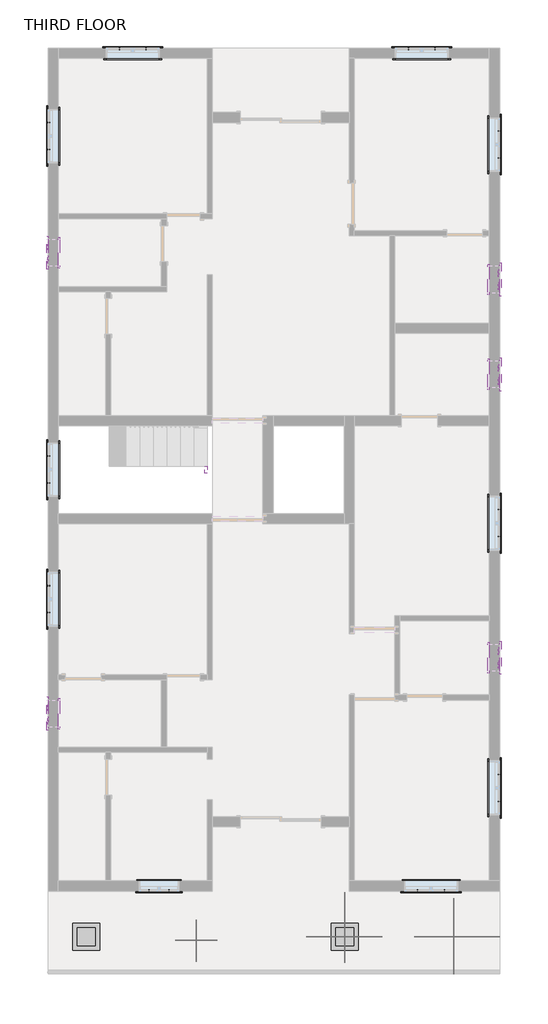
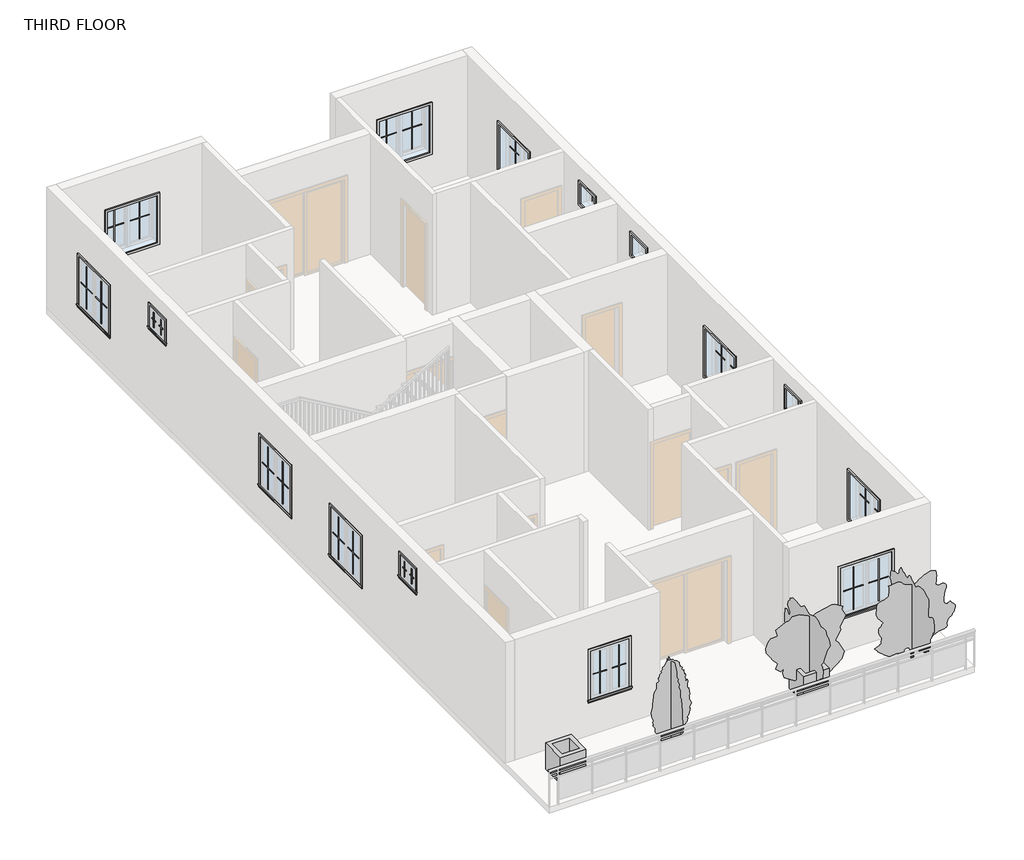
# One storey, part 4 of 4: 60 proxies, 5 geographic elements, 1 railing.
"""IFC4 building model written with IfcOpenShell, lengths in millimetres."""

from ifc_helpers import new_model, si_unit, frame, origin, place, context, project, spatial, polyline, outline, extrude, transform, mapped, element, save
from components import muntin_pattern_2x2_muntin_pattern_2x2_4dfeb3f3, muntin_pattern_2x2_muntin_pattern_2x2_e852a7e4, muntin_pattern_2x2_muntin_pattern_2x2_1acec82f, muntin_pattern_2x2_muntin_pattern_2x2_43d02eee, muntin_pattern_2x2_muntin_pattern_2x2_653c8599, muntin_pattern_2x2_muntin_pattern_2x2_c179cf80, trim_window_exterior_flat_with_sill_7cfdd449, trim_window_exterior_flat_with_sill_e4b28ec3, trim_window_exterior_flat_with_sill_e6f34eb5, trim_window_interior_flat_picture_frame_f1e0b15b, trim_window_interior_flat_picture_frame_39ff4276, trim_window_interior_flat_picture_frame_9a74d23d, planter_2_x2_5b049b04, rpc_tree_conifer_chinese_juniper_7_2_1b9786cd, rpc_tree_fall_american_beech_20_7ed35302, rpc_tree_fall_service_berry_25_c2e4521a

model = new_model("IFC4")

# Units and contexts
model_context = context("Model", 3, world=origin())
ifc_project = project(units=[si_unit("LENGTHUNIT", "METRE", prefix="MILLI")], contexts=[model_context])

# Site, building, storey
site = spatial("IfcSite", under=ifc_project)
building = spatial("IfcBuilding", under=site)
storey = spatial("IfcBuildingStorey", under=building, Name="THIRD FLOOR", Elevation=9601.2)

# Proxies
placement = place(None, origin())
muntin_pattern_2x2_muntin_pattern_2x2_shape = muntin_pattern_2x2_muntin_pattern_2x2_4dfeb3f3(model_context)
element("IfcBuildingElementProxy", 1, Name="Muntin Pattern_2x2 : Muntin Pattern_2x2", ObjectType="Muntin Pattern_2x2 : Muntin Pattern_2x2", at=placement, inside=storey, context=model_context, shape_type="MappedRepresentation", body=[
    mapped(muntin_pattern_2x2_muntin_pattern_2x2_shape, transform((-4756.4414041, 10049.2903263, 10585.45), x_axis=(1.0, 0.0, 0.0), y_axis=(0.0, 1.0, 0.0), z_axis=(0.0, 0.0, 1.0))),
])
element("IfcBuildingElementProxy", 2, Name="Muntin Pattern_2x2 : Muntin Pattern_2x2", ObjectType="Muntin Pattern_2x2 : Muntin Pattern_2x2", at=placement, inside=storey, context=model_context, shape_type="MappedRepresentation", body=[
    mapped(muntin_pattern_2x2_muntin_pattern_2x2_shape, transform((-6348.7039041, 7774.4028263, 10585.45), x_axis=(0.0, 1.0, 0.0), y_axis=(-1.0, 0.0, 0.0), z_axis=(0.0, 0.0, 1.0))),
])
element("IfcBuildingElementProxy", 3, Name="Muntin Pattern_2x2 : Muntin Pattern_2x2", ObjectType="Muntin Pattern_2x2 : Muntin Pattern_2x2", at=placement, inside=storey, context=model_context, shape_type="MappedRepresentation", body=[
    mapped(muntin_pattern_2x2_muntin_pattern_2x2_shape, transform((-6348.7039041, -2664.9971737, 10585.45), x_axis=(0.0, 1.0, 0.0), y_axis=(-1.0, 0.0, 0.0), z_axis=(0.0, 0.0, 1.0))),
])
element("IfcBuildingElementProxy", 4, Name="Muntin Pattern_2x2 : Muntin Pattern_2x2", ObjectType="Muntin Pattern_2x2 : Muntin Pattern_2x2", at=placement, inside=storey, context=model_context, shape_type="MappedRepresentation", body=[
    mapped(muntin_pattern_2x2_muntin_pattern_2x2_shape, transform((2575.0232801, -8930.8596737, 10585.45), x_axis=(-1.0, 0.0, 0.0), y_axis=(0.0, -1.0, 0.0), z_axis=(0.0, 0.0, 1.0))),
])
element("IfcBuildingElementProxy", 5, Name="Muntin Pattern_2x2 : Muntin Pattern_2x2", ObjectType="Muntin Pattern_2x2 : Muntin Pattern_2x2", at=placement, inside=storey, context=model_context, shape_type="MappedRepresentation", body=[
    mapped(muntin_pattern_2x2_muntin_pattern_2x2_shape, transform((3804.9460959, -6313.0721737, 10585.45), x_axis=(0.0, -1.0, 0.0), y_axis=(1.0, 0.0, 0.0), z_axis=(0.0, 0.0, 1.0))),
])
element("IfcBuildingElementProxy", 6, Name="Muntin Pattern_2x2 : Muntin Pattern_2x2", ObjectType="Muntin Pattern_2x2 : Muntin Pattern_2x2", at=placement, inside=storey, context=model_context, shape_type="MappedRepresentation", body=[
    mapped(muntin_pattern_2x2_muntin_pattern_2x2_shape, transform((3804.9460959, -344.0721737, 10585.45), x_axis=(0.0, -1.0, 0.0), y_axis=(1.0, 0.0, 0.0), z_axis=(0.0, 0.0, 1.0))),
])
element("IfcBuildingElementProxy", 7, Name="Muntin Pattern_2x2 : Muntin Pattern_2x2", ObjectType="Muntin Pattern_2x2 : Muntin Pattern_2x2", at=placement, inside=storey, context=model_context, shape_type="MappedRepresentation", body=[
    mapped(muntin_pattern_2x2_muntin_pattern_2x2_shape, transform((3804.9460959, 8190.3278263, 10585.45), x_axis=(0.0, -1.0, 0.0), y_axis=(1.0, 0.0, 0.0), z_axis=(0.0, 0.0, 1.0))),
])
element("IfcBuildingElementProxy", 8, Name="Muntin Pattern_2x2 : Muntin Pattern_2x2", ObjectType="Muntin Pattern_2x2 : Muntin Pattern_2x2", at=placement, inside=storey, context=model_context, shape_type="MappedRepresentation", body=[
    mapped(muntin_pattern_2x2_muntin_pattern_2x2_shape, transform((1758.6585959, 10049.2903263, 10585.45), x_axis=(1.0, 0.0, 0.0), y_axis=(0.0, 1.0, 0.0), z_axis=(0.0, 0.0, 1.0))),
])
element("IfcBuildingElementProxy", 9, Name="Muntin Pattern_2x2 : Muntin Pattern_2x2", ObjectType="Muntin Pattern_2x2 : Muntin Pattern_2x2", at=placement, inside=storey, context=model_context, shape_type="MappedRepresentation", body=[
    mapped(muntin_pattern_2x2_muntin_pattern_2x2_shape, transform((-6348.7039041, 256.0028263, 10585.45), x_axis=(0.0, 1.0, 0.0), y_axis=(-1.0, 0.0, 0.0), z_axis=(0.0, 0.0, 1.0))),
])
muntin_pattern_2x2_muntin_pattern_2x2_2_shape = muntin_pattern_2x2_muntin_pattern_2x2_e852a7e4(model_context)
element("IfcBuildingElementProxy", 10, Name="Muntin Pattern_2x2 : Muntin Pattern_2x2", ObjectType="Muntin Pattern_2x2 : Muntin Pattern_2x2", at=placement, inside=storey, context=model_context, shape_type="MappedRepresentation", body=[
    mapped(muntin_pattern_2x2_muntin_pattern_2x2_2_shape, transform((-4150.0164041, 10049.2903263, 10585.45), x_axis=(-1.0, 0.0, 0.0), y_axis=(0.0, -1.0, 0.0), z_axis=(0.0, 0.0, 1.0))),
])
element("IfcBuildingElementProxy", 11, Name="Muntin Pattern_2x2 : Muntin Pattern_2x2", ObjectType="Muntin Pattern_2x2 : Muntin Pattern_2x2", at=placement, inside=storey, context=model_context, shape_type="MappedRepresentation", body=[
    mapped(muntin_pattern_2x2_muntin_pattern_2x2_2_shape, transform((-6348.7039041, 8380.8278263, 10585.45), x_axis=(0.0, -1.0, 0.0), y_axis=(1.0, 0.0, 0.0), z_axis=(0.0, 0.0, 1.0))),
])
element("IfcBuildingElementProxy", 12, Name="Muntin Pattern_2x2 : Muntin Pattern_2x2", ObjectType="Muntin Pattern_2x2 : Muntin Pattern_2x2", at=placement, inside=storey, context=model_context, shape_type="MappedRepresentation", body=[
    mapped(muntin_pattern_2x2_muntin_pattern_2x2_2_shape, transform((-6348.7039041, -2058.5721737, 10585.45), x_axis=(0.0, -1.0, 0.0), y_axis=(1.0, 0.0, 0.0), z_axis=(0.0, 0.0, 1.0))),
])
element("IfcBuildingElementProxy", 13, Name="Muntin Pattern_2x2 : Muntin Pattern_2x2", ObjectType="Muntin Pattern_2x2 : Muntin Pattern_2x2", at=placement, inside=storey, context=model_context, shape_type="MappedRepresentation", body=[
    mapped(muntin_pattern_2x2_muntin_pattern_2x2_2_shape, transform((1968.5982801, -8930.8596737, 10585.45), x_axis=(1.0, 0.0, 0.0), y_axis=(0.0, 1.0, 0.0), z_axis=(0.0, 0.0, 1.0))),
])
element("IfcBuildingElementProxy", 14, Name="Muntin Pattern_2x2 : Muntin Pattern_2x2", ObjectType="Muntin Pattern_2x2 : Muntin Pattern_2x2", at=placement, inside=storey, context=model_context, shape_type="MappedRepresentation", body=[
    mapped(muntin_pattern_2x2_muntin_pattern_2x2_2_shape, transform((3804.9460959, -6919.4971737, 10585.45), x_axis=(0.0, 1.0, 0.0), y_axis=(-1.0, 0.0, 0.0), z_axis=(0.0, 0.0, 1.0))),
])
element("IfcBuildingElementProxy", 15, Name="Muntin Pattern_2x2 : Muntin Pattern_2x2", ObjectType="Muntin Pattern_2x2 : Muntin Pattern_2x2", at=placement, inside=storey, context=model_context, shape_type="MappedRepresentation", body=[
    mapped(muntin_pattern_2x2_muntin_pattern_2x2_2_shape, transform((3804.9460959, -950.4971737, 10585.45), x_axis=(0.0, 1.0, 0.0), y_axis=(-1.0, 0.0, 0.0), z_axis=(0.0, 0.0, 1.0))),
])
element("IfcBuildingElementProxy", 16, Name="Muntin Pattern_2x2 : Muntin Pattern_2x2", ObjectType="Muntin Pattern_2x2 : Muntin Pattern_2x2", at=placement, inside=storey, context=model_context, shape_type="MappedRepresentation", body=[
    mapped(muntin_pattern_2x2_muntin_pattern_2x2_2_shape, transform((3804.9460959, 7583.9028263, 10585.45), x_axis=(0.0, 1.0, 0.0), y_axis=(-1.0, 0.0, 0.0), z_axis=(0.0, 0.0, 1.0))),
])
element("IfcBuildingElementProxy", 17, Name="Muntin Pattern_2x2 : Muntin Pattern_2x2", ObjectType="Muntin Pattern_2x2 : Muntin Pattern_2x2", at=placement, inside=storey, context=model_context, shape_type="MappedRepresentation", body=[
    mapped(muntin_pattern_2x2_muntin_pattern_2x2_2_shape, transform((2365.0835959, 10049.2903263, 10585.45), x_axis=(-1.0, 0.0, 0.0), y_axis=(0.0, -1.0, 0.0), z_axis=(0.0, 0.0, 1.0))),
])
element("IfcBuildingElementProxy", 18, Name="Muntin Pattern_2x2 : Muntin Pattern_2x2", ObjectType="Muntin Pattern_2x2 : Muntin Pattern_2x2", at=placement, inside=storey, context=model_context, shape_type="MappedRepresentation", body=[
    mapped(muntin_pattern_2x2_muntin_pattern_2x2_2_shape, transform((-6348.7039041, 862.4278263, 10585.45), x_axis=(0.0, -1.0, 0.0), y_axis=(1.0, 0.0, 0.0), z_axis=(0.0, 0.0, 1.0))),
])
muntin_pattern_2x2_muntin_pattern_2x2_3_shape = muntin_pattern_2x2_muntin_pattern_2x2_1acec82f(model_context)
element("IfcBuildingElementProxy", 19, Name="Muntin Pattern_2x2 : Muntin Pattern_2x2", ObjectType="Muntin Pattern_2x2 : Muntin Pattern_2x2", at=placement, inside=storey, context=model_context, shape_type="MappedRepresentation", body=[
    mapped(muntin_pattern_2x2_muntin_pattern_2x2_3_shape, transform((-3635.6664041, -8930.8596737, 10585.45), x_axis=(-1.0, 0.0, 0.0), y_axis=(0.0, -1.0, 0.0), z_axis=(0.0, 0.0, 1.0))),
])
muntin_pattern_2x2_muntin_pattern_2x2_4_shape = muntin_pattern_2x2_muntin_pattern_2x2_43d02eee(model_context)
element("IfcBuildingElementProxy", 20, Name="Muntin Pattern_2x2 : Muntin Pattern_2x2", ObjectType="Muntin Pattern_2x2 : Muntin Pattern_2x2", at=placement, inside=storey, context=model_context, shape_type="MappedRepresentation", body=[
    mapped(muntin_pattern_2x2_muntin_pattern_2x2_4_shape, transform((-4089.6914041, -8930.8596737, 10585.45), x_axis=(1.0, 0.0, 0.0), y_axis=(0.0, 1.0, 0.0), z_axis=(0.0, 0.0, 1.0))),
])
muntin_pattern_2x2_muntin_pattern_2x2_5_shape = muntin_pattern_2x2_muntin_pattern_2x2_653c8599(model_context)
element("IfcBuildingElementProxy", 21, Name="Muntin Pattern_2x2 : Muntin Pattern_2x2", ObjectType="Muntin Pattern_2x2 : Muntin Pattern_2x2", at=placement, inside=storey, context=model_context, shape_type="MappedRepresentation", body=[
    mapped(muntin_pattern_2x2_muntin_pattern_2x2_5_shape, transform((-6348.7039041, 5297.9028263, 11804.65), x_axis=(0.0, 1.0, 0.0), y_axis=(-1.0, 0.0, 0.0), z_axis=(0.0, 0.0, 1.0))),
])
element("IfcBuildingElementProxy", 22, Name="Muntin Pattern_2x2 : Muntin Pattern_2x2", ObjectType="Muntin Pattern_2x2 : Muntin Pattern_2x2", at=placement, inside=storey, context=model_context, shape_type="MappedRepresentation", body=[
    mapped(muntin_pattern_2x2_muntin_pattern_2x2_5_shape, transform((-6348.7039041, -5090.6971737, 11804.65), x_axis=(0.0, 1.0, 0.0), y_axis=(-1.0, 0.0, 0.0), z_axis=(0.0, 0.0, 1.0))),
])
element("IfcBuildingElementProxy", 23, Name="Muntin Pattern_2x2 : Muntin Pattern_2x2", ObjectType="Muntin Pattern_2x2 : Muntin Pattern_2x2", at=placement, inside=storey, context=model_context, shape_type="MappedRepresentation", body=[
    mapped(muntin_pattern_2x2_muntin_pattern_2x2_5_shape, transform((3804.9460959, -3531.7721737, 11804.65), x_axis=(0.0, -1.0, 0.0), y_axis=(1.0, 0.0, 0.0), z_axis=(0.0, 0.0, 1.0))),
])
element("IfcBuildingElementProxy", 24, Name="Muntin Pattern_2x2 : Muntin Pattern_2x2", ObjectType="Muntin Pattern_2x2 : Muntin Pattern_2x2", at=placement, inside=storey, context=model_context, shape_type="MappedRepresentation", body=[
    mapped(muntin_pattern_2x2_muntin_pattern_2x2_5_shape, transform((3804.9460959, 2856.3278263, 11804.65), x_axis=(0.0, -1.0, 0.0), y_axis=(1.0, 0.0, 0.0), z_axis=(0.0, 0.0, 1.0))),
])
element("IfcBuildingElementProxy", 25, Name="Muntin Pattern_2x2 : Muntin Pattern_2x2", ObjectType="Muntin Pattern_2x2 : Muntin Pattern_2x2", at=placement, inside=storey, context=model_context, shape_type="MappedRepresentation", body=[
    mapped(muntin_pattern_2x2_muntin_pattern_2x2_5_shape, transform((3804.9460959, 4996.2778263, 11804.65), x_axis=(0.0, -1.0, 0.0), y_axis=(1.0, 0.0, 0.0), z_axis=(0.0, 0.0, 1.0))),
])
muntin_pattern_2x2_muntin_pattern_2x2_6_shape = muntin_pattern_2x2_muntin_pattern_2x2_c179cf80(model_context)
element("IfcBuildingElementProxy", 26, Name="Muntin Pattern_2x2 : Muntin Pattern_2x2", ObjectType="Muntin Pattern_2x2 : Muntin Pattern_2x2", at=placement, inside=storey, context=model_context, shape_type="MappedRepresentation", body=[
    mapped(muntin_pattern_2x2_muntin_pattern_2x2_6_shape, transform((-6348.7039041, 5599.5278263, 11804.65), x_axis=(0.0, -1.0, 0.0), y_axis=(1.0, 0.0, 0.0), z_axis=(0.0, 0.0, 1.0))),
])
element("IfcBuildingElementProxy", 27, Name="Muntin Pattern_2x2 : Muntin Pattern_2x2", ObjectType="Muntin Pattern_2x2 : Muntin Pattern_2x2", at=placement, inside=storey, context=model_context, shape_type="MappedRepresentation", body=[
    mapped(muntin_pattern_2x2_muntin_pattern_2x2_6_shape, transform((-6348.7039041, -4789.0721737, 11804.65), x_axis=(0.0, -1.0, 0.0), y_axis=(1.0, 0.0, 0.0), z_axis=(0.0, 0.0, 1.0))),
])
element("IfcBuildingElementProxy", 28, Name="Muntin Pattern_2x2 : Muntin Pattern_2x2", ObjectType="Muntin Pattern_2x2 : Muntin Pattern_2x2", at=placement, inside=storey, context=model_context, shape_type="MappedRepresentation", body=[
    mapped(muntin_pattern_2x2_muntin_pattern_2x2_6_shape, transform((3804.9460959, -3833.3971737, 11804.65), x_axis=(0.0, 1.0, 0.0), y_axis=(-1.0, 0.0, 0.0), z_axis=(0.0, 0.0, 1.0))),
])
element("IfcBuildingElementProxy", 29, Name="Muntin Pattern_2x2 : Muntin Pattern_2x2", ObjectType="Muntin Pattern_2x2 : Muntin Pattern_2x2", at=placement, inside=storey, context=model_context, shape_type="MappedRepresentation", body=[
    mapped(muntin_pattern_2x2_muntin_pattern_2x2_6_shape, transform((3804.9460959, 2554.7028263, 11804.65), x_axis=(0.0, 1.0, 0.0), y_axis=(-1.0, 0.0, 0.0), z_axis=(0.0, 0.0, 1.0))),
])
element("IfcBuildingElementProxy", 30, Name="Muntin Pattern_2x2 : Muntin Pattern_2x2", ObjectType="Muntin Pattern_2x2 : Muntin Pattern_2x2", at=placement, inside=storey, context=model_context, shape_type="MappedRepresentation", body=[
    mapped(muntin_pattern_2x2_muntin_pattern_2x2_6_shape, transform((3804.9460959, 4694.6528263, 11804.65), x_axis=(0.0, 1.0, 0.0), y_axis=(-1.0, 0.0, 0.0), z_axis=(0.0, 0.0, 1.0))),
])
trim_window_exterior_flat_with_sill_shape = trim_window_exterior_flat_with_sill_7cfdd449(model_context)
element("IfcBuildingElementProxy", 31, Name="Trim-Window-Exterior-Flat : with Sill", ObjectType="Trim-Window-Exterior-Flat : with Sill", at=placement, inside=storey, context=model_context, shape_type="MappedRepresentation", body=[
    mapped(trim_window_exterior_flat_with_sill_shape, transform((-4453.2289041, 10058.8153263, 11734.8), x_axis=(-1.0, 0.0, 0.0), y_axis=(0.0, 0.0, 1.0), z_axis=(0.0, 1.0, 0.0))),
])
element("IfcBuildingElementProxy", 32, Name="Trim-Window-Exterior-Flat : with Sill", ObjectType="Trim-Window-Exterior-Flat : with Sill", at=placement, inside=storey, context=model_context, shape_type="MappedRepresentation", body=[
    mapped(trim_window_exterior_flat_with_sill_shape, transform((-6358.2289041, 8077.6153263, 11734.8), x_axis=(0.0, -1.0, 0.0), y_axis=(0.0, 0.0, 1.0), z_axis=(-1.0, 0.0, 0.0))),
])
element("IfcBuildingElementProxy", 33, Name="Trim-Window-Exterior-Flat : with Sill", ObjectType="Trim-Window-Exterior-Flat : with Sill", at=placement, inside=storey, context=model_context, shape_type="MappedRepresentation", body=[
    mapped(trim_window_exterior_flat_with_sill_shape, transform((-6358.2289041, -2361.7846737, 11734.8), x_axis=(0.0, -1.0, 0.0), y_axis=(0.0, 0.0, 1.0), z_axis=(-1.0, 0.0, 0.0))),
])
element("IfcBuildingElementProxy", 34, Name="Trim-Window-Exterior-Flat : with Sill", ObjectType="Trim-Window-Exterior-Flat : with Sill", at=placement, inside=storey, context=model_context, shape_type="MappedRepresentation", body=[
    mapped(trim_window_exterior_flat_with_sill_shape, transform((2271.8107801, -8940.3846737, 11734.8), x_axis=(1.0, 0.0, 0.0), y_axis=(0.0, 0.0, 1.0), z_axis=(0.0, -1.0, 0.0))),
])
element("IfcBuildingElementProxy", 35, Name="Trim-Window-Exterior-Flat : with Sill", ObjectType="Trim-Window-Exterior-Flat : with Sill", at=placement, inside=storey, context=model_context, shape_type="MappedRepresentation", body=[
    mapped(trim_window_exterior_flat_with_sill_shape, transform((3814.4710959, -6616.2846737, 11734.8), x_axis=(0.0, 1.0, 0.0), y_axis=(0.0, 0.0, 1.0), z_axis=(1.0, 0.0, 0.0))),
])
element("IfcBuildingElementProxy", 36, Name="Trim-Window-Exterior-Flat : with Sill", ObjectType="Trim-Window-Exterior-Flat : with Sill", at=placement, inside=storey, context=model_context, shape_type="MappedRepresentation", body=[
    mapped(trim_window_exterior_flat_with_sill_shape, transform((3814.4710959, -647.2846737, 11734.8), x_axis=(0.0, 1.0, 0.0), y_axis=(0.0, 0.0, 1.0), z_axis=(1.0, 0.0, 0.0))),
])
element("IfcBuildingElementProxy", 37, Name="Trim-Window-Exterior-Flat : with Sill", ObjectType="Trim-Window-Exterior-Flat : with Sill", at=placement, inside=storey, context=model_context, shape_type="MappedRepresentation", body=[
    mapped(trim_window_exterior_flat_with_sill_shape, transform((3814.4710959, 7887.1153263, 11734.8), x_axis=(0.0, 1.0, 0.0), y_axis=(0.0, 0.0, 1.0), z_axis=(1.0, 0.0, 0.0))),
])
element("IfcBuildingElementProxy", 38, Name="Trim-Window-Exterior-Flat : with Sill", ObjectType="Trim-Window-Exterior-Flat : with Sill", at=placement, inside=storey, context=model_context, shape_type="MappedRepresentation", body=[
    mapped(trim_window_exterior_flat_with_sill_shape, transform((2061.8710959, 10058.8153263, 11734.8), x_axis=(-1.0, 0.0, 0.0), y_axis=(0.0, 0.0, 1.0), z_axis=(0.0, 1.0, 0.0))),
])
element("IfcBuildingElementProxy", 39, Name="Trim-Window-Exterior-Flat : with Sill", ObjectType="Trim-Window-Exterior-Flat : with Sill", at=placement, inside=storey, context=model_context, shape_type="MappedRepresentation", body=[
    mapped(trim_window_exterior_flat_with_sill_shape, transform((-6358.2289041, 559.2153263, 11734.8), x_axis=(0.0, -1.0, 0.0), y_axis=(0.0, 0.0, 1.0), z_axis=(-1.0, 0.0, 0.0))),
])
trim_window_exterior_flat_with_sill_2_shape = trim_window_exterior_flat_with_sill_e4b28ec3(model_context)
element("IfcBuildingElementProxy", 40, Name="Trim-Window-Exterior-Flat : with Sill", ObjectType="Trim-Window-Exterior-Flat : with Sill", at=placement, inside=storey, context=model_context, shape_type="MappedRepresentation", body=[
    mapped(trim_window_exterior_flat_with_sill_2_shape, transform((-3862.6789041, -8940.3846737, 11734.8), x_axis=(1.0, 0.0, 0.0), y_axis=(0.0, 0.0, 1.0), z_axis=(0.0, -1.0, 0.0))),
])
trim_window_exterior_flat_with_sill_3_shape = trim_window_exterior_flat_with_sill_e6f34eb5(model_context)
element("IfcBuildingElementProxy", 41, Name="Trim-Window-Exterior-Flat : with Sill", ObjectType="Trim-Window-Exterior-Flat : with Sill", at=placement, inside=storey, context=model_context, shape_type="MappedRepresentation", body=[
    mapped(trim_window_exterior_flat_with_sill_3_shape, transform((-6358.2289041, 5448.7153263, 12268.2), x_axis=(0.0, -1.0, 0.0), y_axis=(0.0, 0.0, 1.0), z_axis=(-1.0, 0.0, 0.0))),
])
element("IfcBuildingElementProxy", 42, Name="Trim-Window-Exterior-Flat : with Sill", ObjectType="Trim-Window-Exterior-Flat : with Sill", at=placement, inside=storey, context=model_context, shape_type="MappedRepresentation", body=[
    mapped(trim_window_exterior_flat_with_sill_3_shape, transform((-6358.2289041, -4939.8846737, 12268.2), x_axis=(0.0, -1.0, 0.0), y_axis=(0.0, 0.0, 1.0), z_axis=(-1.0, 0.0, 0.0))),
])
element("IfcBuildingElementProxy", 43, Name="Trim-Window-Exterior-Flat : with Sill", ObjectType="Trim-Window-Exterior-Flat : with Sill", at=placement, inside=storey, context=model_context, shape_type="MappedRepresentation", body=[
    mapped(trim_window_exterior_flat_with_sill_3_shape, transform((3814.4710959, -3682.5846737, 12268.2), x_axis=(0.0, 1.0, 0.0), y_axis=(0.0, 0.0, 1.0), z_axis=(1.0, 0.0, 0.0))),
])
element("IfcBuildingElementProxy", 44, Name="Trim-Window-Exterior-Flat : with Sill", ObjectType="Trim-Window-Exterior-Flat : with Sill", at=placement, inside=storey, context=model_context, shape_type="MappedRepresentation", body=[
    mapped(trim_window_exterior_flat_with_sill_3_shape, transform((3814.4710959, 2705.5153263, 12268.2), x_axis=(0.0, 1.0, 0.0), y_axis=(0.0, 0.0, 1.0), z_axis=(1.0, 0.0, 0.0))),
])
element("IfcBuildingElementProxy", 45, Name="Trim-Window-Exterior-Flat : with Sill", ObjectType="Trim-Window-Exterior-Flat : with Sill", at=placement, inside=storey, context=model_context, shape_type="MappedRepresentation", body=[
    mapped(trim_window_exterior_flat_with_sill_3_shape, transform((3814.4710959, 4845.4653263, 12268.2), x_axis=(0.0, 1.0, 0.0), y_axis=(0.0, 0.0, 1.0), z_axis=(1.0, 0.0, 0.0))),
])
trim_window_interior_flat_picture_frame_shape = trim_window_interior_flat_picture_frame_f1e0b15b(model_context)
element("IfcBuildingElementProxy", 46, Name="Trim-Window-Interior-Flat : Picture Frame", ObjectType="Trim-Window-Interior-Flat : Picture Frame", at=placement, inside=storey, context=model_context, shape_type="MappedRepresentation", body=[
    mapped(trim_window_interior_flat_picture_frame_shape, transform((-4453.2289041, 9830.2153263, 11734.8), x_axis=(1.0, 0.0, 0.0), y_axis=(0.0, 0.0, 1.0), z_axis=(0.0, -1.0, 0.0))),
])
element("IfcBuildingElementProxy", 47, Name="Trim-Window-Interior-Flat : Picture Frame", ObjectType="Trim-Window-Interior-Flat : Picture Frame", at=placement, inside=storey, context=model_context, shape_type="MappedRepresentation", body=[
    mapped(trim_window_interior_flat_picture_frame_shape, transform((-6129.6289041, 8077.6153263, 11734.8), x_axis=(0.0, 1.0, 0.0), y_axis=(0.0, 0.0, 1.0), z_axis=(1.0, 0.0, 0.0))),
])
element("IfcBuildingElementProxy", 48, Name="Trim-Window-Interior-Flat : Picture Frame", ObjectType="Trim-Window-Interior-Flat : Picture Frame", at=placement, inside=storey, context=model_context, shape_type="MappedRepresentation", body=[
    mapped(trim_window_interior_flat_picture_frame_shape, transform((-6129.6289041, -2361.7846737, 11734.8), x_axis=(0.0, 1.0, 0.0), y_axis=(0.0, 0.0, 1.0), z_axis=(1.0, 0.0, 0.0))),
])
element("IfcBuildingElementProxy", 49, Name="Trim-Window-Interior-Flat : Picture Frame", ObjectType="Trim-Window-Interior-Flat : Picture Frame", at=placement, inside=storey, context=model_context, shape_type="MappedRepresentation", body=[
    mapped(trim_window_interior_flat_picture_frame_shape, transform((2271.8107801, -8711.7846737, 11734.8), x_axis=(-1.0, 0.0, 0.0), y_axis=(0.0, 0.0, 1.0), z_axis=(0.0, 1.0, 0.0))),
])
element("IfcBuildingElementProxy", 50, Name="Trim-Window-Interior-Flat : Picture Frame", ObjectType="Trim-Window-Interior-Flat : Picture Frame", at=placement, inside=storey, context=model_context, shape_type="MappedRepresentation", body=[
    mapped(trim_window_interior_flat_picture_frame_shape, transform((3585.8710959, -6616.2846737, 11734.8), x_axis=(0.0, -1.0, 0.0), y_axis=(0.0, 0.0, 1.0), z_axis=(-1.0, 0.0, 0.0))),
])
element("IfcBuildingElementProxy", 51, Name="Trim-Window-Interior-Flat : Picture Frame", ObjectType="Trim-Window-Interior-Flat : Picture Frame", at=placement, inside=storey, context=model_context, shape_type="MappedRepresentation", body=[
    mapped(trim_window_interior_flat_picture_frame_shape, transform((3585.8710959, -647.2846737, 11734.8), x_axis=(0.0, -1.0, 0.0), y_axis=(0.0, 0.0, 1.0), z_axis=(-1.0, 0.0, 0.0))),
])
element("IfcBuildingElementProxy", 52, Name="Trim-Window-Interior-Flat : Picture Frame", ObjectType="Trim-Window-Interior-Flat : Picture Frame", at=placement, inside=storey, context=model_context, shape_type="MappedRepresentation", body=[
    mapped(trim_window_interior_flat_picture_frame_shape, transform((3585.8710959, 7887.1153263, 11734.8), x_axis=(0.0, -1.0, 0.0), y_axis=(0.0, 0.0, 1.0), z_axis=(-1.0, 0.0, 0.0))),
])
element("IfcBuildingElementProxy", 53, Name="Trim-Window-Interior-Flat : Picture Frame", ObjectType="Trim-Window-Interior-Flat : Picture Frame", at=placement, inside=storey, context=model_context, shape_type="MappedRepresentation", body=[
    mapped(trim_window_interior_flat_picture_frame_shape, transform((2061.8710959, 9830.2153263, 11734.8), x_axis=(1.0, 0.0, 0.0), y_axis=(0.0, 0.0, 1.0), z_axis=(0.0, -1.0, 0.0))),
])
element("IfcBuildingElementProxy", 54, Name="Trim-Window-Interior-Flat : Picture Frame", ObjectType="Trim-Window-Interior-Flat : Picture Frame", at=placement, inside=storey, context=model_context, shape_type="MappedRepresentation", body=[
    mapped(trim_window_interior_flat_picture_frame_shape, transform((-6129.6289041, 559.2153263, 11734.8), x_axis=(0.0, 1.0, 0.0), y_axis=(0.0, 0.0, 1.0), z_axis=(1.0, 0.0, 0.0))),
])
trim_window_interior_flat_picture_frame_2_shape = trim_window_interior_flat_picture_frame_39ff4276(model_context)
element("IfcBuildingElementProxy", 55, Name="Trim-Window-Interior-Flat : Picture Frame", ObjectType="Trim-Window-Interior-Flat : Picture Frame", at=placement, inside=storey, context=model_context, shape_type="MappedRepresentation", body=[
    mapped(trim_window_interior_flat_picture_frame_2_shape, transform((-3862.6789041, -8711.7846737, 11734.8), x_axis=(-1.0, 0.0, 0.0), y_axis=(0.0, 0.0, 1.0), z_axis=(0.0, 1.0, 0.0))),
])
trim_window_interior_flat_picture_frame_3_shape = trim_window_interior_flat_picture_frame_9a74d23d(model_context)
element("IfcBuildingElementProxy", 56, Name="Trim-Window-Interior-Flat : Picture Frame", ObjectType="Trim-Window-Interior-Flat : Picture Frame", at=placement, inside=storey, context=model_context, shape_type="MappedRepresentation", body=[
    mapped(trim_window_interior_flat_picture_frame_3_shape, transform((-6129.6289041, 5448.7153263, 12268.2), x_axis=(0.0, 1.0, 0.0), y_axis=(0.0, 0.0, 1.0), z_axis=(1.0, 0.0, 0.0))),
])
element("IfcBuildingElementProxy", 57, Name="Trim-Window-Interior-Flat : Picture Frame", ObjectType="Trim-Window-Interior-Flat : Picture Frame", at=placement, inside=storey, context=model_context, shape_type="MappedRepresentation", body=[
    mapped(trim_window_interior_flat_picture_frame_3_shape, transform((-6129.6289041, -4939.8846737, 12268.2), x_axis=(0.0, 1.0, 0.0), y_axis=(0.0, 0.0, 1.0), z_axis=(1.0, 0.0, 0.0))),
])
element("IfcBuildingElementProxy", 58, Name="Trim-Window-Interior-Flat : Picture Frame", ObjectType="Trim-Window-Interior-Flat : Picture Frame", at=placement, inside=storey, context=model_context, shape_type="MappedRepresentation", body=[
    mapped(trim_window_interior_flat_picture_frame_3_shape, transform((3585.8710959, -3682.5846737, 12268.2), x_axis=(0.0, -1.0, 0.0), y_axis=(0.0, 0.0, 1.0), z_axis=(-1.0, 0.0, 0.0))),
])
element("IfcBuildingElementProxy", 59, Name="Trim-Window-Interior-Flat : Picture Frame", ObjectType="Trim-Window-Interior-Flat : Picture Frame", at=placement, inside=storey, context=model_context, shape_type="MappedRepresentation", body=[
    mapped(trim_window_interior_flat_picture_frame_3_shape, transform((3585.8710959, 2705.5153263, 12268.2), x_axis=(0.0, -1.0, 0.0), y_axis=(0.0, 0.0, 1.0), z_axis=(-1.0, 0.0, 0.0))),
])
element("IfcBuildingElementProxy", 60, Name="Trim-Window-Interior-Flat : Picture Frame", ObjectType="Trim-Window-Interior-Flat : Picture Frame", at=placement, inside=storey, context=model_context, shape_type="MappedRepresentation", body=[
    mapped(trim_window_interior_flat_picture_frame_3_shape, transform((3585.8710959, 4845.4653263, 12268.2), x_axis=(0.0, -1.0, 0.0), y_axis=(0.0, 0.0, 1.0), z_axis=(-1.0, 0.0, 0.0))),
])

# Geographic elements
planter_2_x2_shape = planter_2_x2_5b049b04(model_context)
element("IfcGeographicElement", 61, ObjectType="Planter : 2'X2'", at=placement, inside=storey, context=model_context, shape_type="MappedRepresentation", body=[
    mapped(planter_2_x2_shape, transform((-5500.9789041, -9969.0846737, 9601.2), x_axis=(1.0, 0.0, 0.0), y_axis=(0.0, 1.0, 0.0), z_axis=(0.0, 0.0, 1.0))),
])
element("IfcGeographicElement", 62, ObjectType="Planter : 2'X2'", at=placement, inside=storey, context=model_context, shape_type="MappedRepresentation", body=[
    mapped(planter_2_x2_shape, transform((328.3210959, -9969.0846737, 9601.2), x_axis=(1.0, 0.0, 0.0), y_axis=(0.0, 1.0, 0.0), z_axis=(0.0, 0.0, 1.0))),
])
rpc_tree_conifer_chinese_juniper_7_2_shape = rpc_tree_conifer_chinese_juniper_7_2_1b9786cd(model_context)
element("IfcGeographicElement", 63, ObjectType="RPC Tree - Conifer : Chinese Juniper - 7' 2", at=placement, inside=storey, context=model_context, shape_type="MappedRepresentation", body=[
    mapped(rpc_tree_conifer_chinese_juniper_7_2_shape, transform((-3024.6755752, -10045.2846737, 9601.2), x_axis=(1.0, 0.0, 0.0), y_axis=(0.0, 1.0, 0.0), z_axis=(0.0, 0.0, 1.0))),
])
rpc_tree_fall_american_beech_20_shape = rpc_tree_fall_american_beech_20_7ed35302(model_context)
element("IfcGeographicElement", 64, ObjectType="RPC Tree - Fall : American Beech - 20'", at=placement, inside=storey, context=model_context, shape_type="MappedRepresentation", body=[
    mapped(rpc_tree_fall_american_beech_20_shape, transform((2785.7710959, -9969.0846737, 9601.2), x_axis=(1.0, 0.0, 0.0), y_axis=(0.0, 1.0, 0.0), z_axis=(0.0, 0.0, 1.0))),
])
rpc_tree_fall_service_berry_25_shape = rpc_tree_fall_service_berry_25_c2e4521a(model_context)
element("IfcGeographicElement", 65, ObjectType="RPC Tree - Fall : Service Berry - 25'", at=placement, inside=storey, context=model_context, shape_type="MappedRepresentation", body=[
    mapped(rpc_tree_fall_service_berry_25_shape, transform((328.3210959, -9969.0846737, 9601.2), x_axis=(1.0, 0.0, 0.0), y_axis=(0.0, 1.0, 0.0), z_axis=(0.0, 0.0, 1.0))),
])

# Railing
element("IfcRailing", 66, ObjectType="Handrail - Rectangular", at=placement, inside=storey, context=model_context, shape_type="SweptSolid", body=[
    extrude(outline(polyline([(-2827.6289041, 635.4153263), (-2776.8289041, 635.4153263), (-2776.8289041, 483.0153263), (-2827.6289041, 483.0153263), (-2827.6289041, 635.4153263)])), frame((0.0, 0.0, 12065.0), z_axis=(0.0, 0.0, 1.0), x_axis=(1.0, 0.0, 0.0)), (0.0, 0.0, 1.0), 50.8),
    extrude(outline(polyline([(-2792.7039041, 543.3403263), (-2792.7039041, 524.2903263), (-2811.7539041, 524.2903263), (-2811.7539041, 543.3403263), (-2792.7039041, 543.3403263)])), frame((0.0, 0.0, 11201.4), z_axis=(0.0, 0.0, 1.0), x_axis=(1.0, 0.0, 0.0)), (0.0, 0.0, 1.0), 863.6),
    extrude(outline(polyline([(-2792.7039041, 502.0653263), (-2792.7039041, 483.0153263), (-2811.7539041, 483.0153263), (-2811.7539041, 502.0653263), (-2792.7039041, 502.0653263)])), frame((0.0, 0.0, 11201.4), z_axis=(0.0, 0.0, 1.0), x_axis=(1.0, 0.0, 0.0)), (0.0, 0.0, 1.0), 863.6),
    extrude(outline(polyline([(-2792.7039041, 635.4153263), (-2792.7039041, 616.3653263), (-2811.7539041, 616.3653263), (-2811.7539041, 635.4153263), (-2792.7039041, 635.4153263)])), frame((0.0, 0.0, 11201.4), z_axis=(0.0, 0.0, 1.0), x_axis=(1.0, 0.0, 0.0)), (0.0, 0.0, 1.0), 863.6),
])

save(model, "model.ifc")

# Revit data of these elements
# Type "Muntin Pattern_2x2 : Muntin Pattern_2x2"
#   Width [instance default] = 4' - 0"
#   Thickness = 0' - 0 1/2"
#   Height [instance default] = 4' - 0"
#   Distance = 0' - 0 3/4"
#   Interior Material [instance default] = none
#   Exterior Material [instance default] = none
#   Default Elevation = 0
# Type "Trim-Window-Exterior-Flat : with Sill"
#   Trim Width = 0' - 2 1/4"
#   Trim Thickness_Picture Frame = 0' - 1 1/4"
#   Trim Thickness_with Sill = 0' - 0 3/4"
#   Sill Thickness = 0' - 1 1/4"
#   Opening Width [instance default] = 2' - 0"
#   Opening Height [instance default] = 3' - 0"
#   Default Elevation = 4' - 0"
#   Sill = yes
#   Picture Frame = no
#   Trim Material [instance default] = none
# Type "Trim-Window-Interior-Flat : Picture Frame"
#   Trim Thickness_Picture Frame = 0' - 1 1/4"
#   Trim Width = 0' - 2 1/4"
#   Trim Thickness_with Sill = 0' - 0 3/4"
#   Sill Thickness = 0' - 1 1/4"
#   Opening Width [instance default] = 2' - 0"
#   Opening Height [instance default] = 3' - 0"
#   Default Elevation = 4' - 0"
#   Sill = no
#   Picture Frame = yes
#   Trim Material [instance default] = none
# Type "Planter : 2'X2'"
#   Depth = 2' - 0"
#   Height = 2' - 6"
#   Width = 2' - 0"
#   Material = Concrete, Precast
# Type "RPC Tree - Conifer : Chinese Juniper - 7' 2"
#   built-in parameter 1005198 = "{2, 15},{39, RPC-16-FUM3-UUQ0-UBF0-N000-ST1L-LVER-AU},{1, 0},{1, 0},{2, 35},{1, 8},{5, Color},{1, 0},{1, 0},{3, 0.8},{3, 0.8},{3, 0.8},{1, 8},{7, BBoxMin},{1, 0},{1, 0},{1, 0},{1, 0},{1, 0},{1, 8},{7, BBoxMax},{1, 0},{1, 0},{1, 0},{1, 0},{1, 0},{2, 11},{9, RPCTypeId},{1, 0},{1, 0},{39, RPC-16-FUM3-UUQ0-UBF0-N000-ST1L-LVER-AU},{1, 6},{14, RPCPlantHeight},{1, 0},{1, 0},{1, 7},{2, 11},{7, keyword},{1, 0},{1, 0},{96, :Geometry:RPC:Chinese Juniper:juniperus chinensis:chinese:juniper:cupressaceae:conifer:evergreen},{2, 11},{8, category},{1, 0},{1, 0},{16, :Trees [General]},{2, 11},{12, LocalizedUID},{1, 0},{1, 0},{15, Chinese Juniper},{2, 14},{6, Height},{1, 0},{1, 0},{1, 7},{1, 2},{16, Cast Reflections},{1, 0},{1, 0},{1, 0},{1, 2},{12, Cast Shadows},{1, 0},{1, 0},{1, 1},{1, 2},{9, Lock View},{1, 0},{1, 0},{1, 0},{1, 4},{5, ViewC},{1, 0},{1, 0},{1, 0},{2, 11},{20, AdvancedUIDefinition},{1, 0},{1, 0},{0, },{2, 11},{10, AssetLibID},{1, 0},{1, 0},{36, 4D3F6E72-3F99-4203-98E9-AF80B3C7A7A4},{2, 11},{10, BaseSchema},{1, 0},{1, 0},{9, RPCSchema},{2, 11},{12, ExchangeGUID},{1, 0},{1, 0},{0, },{1, 2},{6, Hidden},{1, 0},{1, 0},{1, 0},{1, 4},{11, RPCCategory},{1, 0},{1, 0},{1, 0},{2, 11},{8, RPCImage},{1, 0},{1, 0},{0, },{1, 4},{13, SchemaVersion},{1, 0},{1, 0},{1, 4},{2, 11},{12, UIDefinition},{1, 0},{1, 0},{0, },{2, 11},{6, UIName},{1, 0},{1, 0},{39, RPC-16-FUM3-UUQ0-UBF0-N000-ST1L-LVER-AU},{2, 11},{11, VersionGUID},{1, 0},{1, 0},{9, RPCSchema},{2, 11},{9, assettype},{1, 0},{1, 0},{11, RPCGeometry},{2, 11},{11, description},{1, 0},{1, 0},{0, },{2, 11},{9, localname},{1, 0},{1, 0},{3, RPC},{2, 11},{9, localtype},{1, 0},{1, 0},{3, RPC},{1, 4},{8, revision},{1, 0},{1, 0},{1, 1},{2, 11},{9, thumbnail},{1, 0},{1, 0},{0, },{1, 4},{7, version},{1, 0},{1, 0},{1, 1},{1, 2},{20, RPC_Cast Reflections},{1, 0},{1, 0},{1, 1},{1, 2},{16, RPC_Cast Shadows},{1, 0},{1, 0},{1, 1},{1, 2},{13, RPC_Lock View},{1, 0},{1, 0},{1, 0},{1, 4},{9, RPC_ViewC},{1, 0},{1, 0},{1, 0},{21, assetlibrary_base.fbx},{1, 5},"
#   built-in parameter 1005195 = "RPC-16-FUM3-UUQ0-UBF0-N000-ST1L-LVER-AU"
#   Type Comments = "Chinese Juniper"
#   Assembly Code = "G2050500"
#   Height = 7' - 0"
#   Description = (empty or 0)
#   Default Elevation = 0
# Type "RPC Tree - Fall : American Beech - 20'"
#   built-in parameter 1005198 = "{2, 15},{39, RPC-16-G2VX-NFFX-5QM5-6000-ST1L-LVER-AU},{1, 0},{1, 0},{2, 13},{1, 8},{5, Color},{1, 0},{1, 0},{3, 0.8},{3, 0.8},{3, 0.8},{1, 8},{7, BBoxMin},{1, 0},{1, 0},{1, 0},{1, 0},{1, 0},{1, 8},{7, BBoxMax},{1, 0},{1, 0},{1, 0},{1, 0},{1, 0},{2, 11},{9, RPCTypeId},{1, 0},{1, 0},{39, RPC-16-G2VX-NFFX-5QM5-6000-ST1L-LVER-AU},{1, 6},{14, RPCPlantHeight},{1, 0},{1, 0},{2, 20},{2, 11},{7, keyword},{1, 0},{1, 0},{39, :RPCs:Fall Trees [General]:Geometry:RPC},{2, 11},{8, category},{1, 0},{1, 0},{20, Fall Trees [General]},{2, 11},{12, LocalizedUID},{1, 0},{1, 0},{21, American Beech [Fall]},{2, 14},{6, Height},{1, 0},{1, 0},{2, 20},{1, 2},{16, Cast Reflections},{1, 0},{1, 0},{1, 0},{1, 2},{12, Cast Shadows},{1, 0},{1, 0},{1, 1},{1, 2},{9, Lock View},{1, 0},{1, 0},{1, 0},{1, 4},{5, ViewC},{1, 0},{1, 0},{1, 0},{21, assetlibrary_base.fbx},{1, 5},"
#   built-in parameter 1005195 = "RPC-16-G2VX-NFFX-5QM5-6000-ST1L-LVER-AU"
#   Type Comments = "American Beech"
#   Assembly Code = "G2050500"
#   Height = 7' - 0"
#   Default Elevation = 0
# Type "RPC Tree - Fall : Service Berry - 25'"
#   built-in parameter 1005198 = "{2, 15},{39, RPC-16-FVGU-8VG0-7PL0-4000-ST1L-LVER-AU},{1, 0},{1, 0},{2, 13},{1, 8},{5, Color},{1, 0},{1, 0},{3, 0.8},{3, 0.8},{3, 0.8},{1, 8},{7, BBoxMin},{1, 0},{1, 0},{1, 0},{1, 0},{1, 0},{1, 8},{7, BBoxMax},{1, 0},{1, 0},{1, 0},{1, 0},{1, 0},{2, 11},{9, RPCTypeId},{1, 0},{1, 0},{39, RPC-16-FVGU-8VG0-7PL0-4000-ST1L-LVER-AU},{1, 6},{14, RPCPlantHeight},{1, 0},{1, 0},{2, 25},{2, 11},{7, keyword},{1, 0},{1, 0},{39, :RPCs:Fall Trees [General]:Geometry:RPC},{2, 11},{8, category},{1, 0},{1, 0},{20, Fall Trees [General]},{2, 11},{12, LocalizedUID},{1, 0},{1, 0},{20, Service Berry [Fall]},{2, 14},{6, Height},{1, 0},{1, 0},{2, 25},{1, 2},{16, Cast Reflections},{1, 0},{1, 0},{1, 0},{1, 2},{12, Cast Shadows},{1, 0},{1, 0},{1, 1},{1, 2},{9, Lock View},{1, 0},{1, 0},{1, 0},{1, 4},{5, ViewC},{1, 0},{1, 0},{1, 0},{21, assetlibrary_base.fbx},{1, 5},"
#   built-in parameter 1005195 = "RPC-16-FVGU-8VG0-7PL0-4000-ST1L-LVER-AU"
#   Type Comments = "Service Berry"
#   Assembly Code = "G2050500"
#   Height = 7' - 0"
#   Default Elevation = 0
# Type "Handrail - Rectangular"
#   Assembly Code = "C2010400"
#   built-in parameter 1008612 = 0.0416667 (stored number, unit not read)
#   built-in parameter 1008611 = 0.0416667 (stored number, unit not read)
#   built-in parameter 1008609 = 0.333333 (stored number, unit not read)
#   built-in parameter 1008604 = 0.166667 (stored number, unit not read)
#   built-in parameter 1008603 = 0.166667 (stored number, unit not read)
#   Railing Height = 3' - 0"
#   built-in parameter 1008630 = 2
#   built-in parameter 1008610 = 2
#   built-in parameter 1008618 = Baluster - Square : 3/4"
# Elements 1, 2, 3, 4, 5, 6, 7, 8, 9, 10, 11, 12, 13, 14, 15, 16, 17, 18 (IfcBuildingElementProxy, "Muntin Pattern_2x2 : Muntin Pattern_2x2")
#   Width = 1' - 6 5/8"
#   Height = 3' - 6 1/2"
#   Interior Material = Wood - Stained
#   Exterior Material = Clad - White
#   Phase Created = New Construction
#   Materials on its faces: "Clad - White", "Wood - Stained"
# Elements 19, 20 (IfcBuildingElementProxy, "Muntin Pattern_2x2 : Muntin Pattern_2x2")
#   Width = 1' - 0 5/8"
#   Height = 3' - 6 1/2"
#   Interior Material = Wood - Stained
#   Exterior Material = Clad - White
#   Phase Created = New Construction
#   Materials on its faces: "Clad - White", "Wood - Stained"
# Elements 21, 22, 23, 24, 25, 26, 27, 28, 29, 30 (IfcBuildingElementProxy, "Muntin Pattern_2x2 : Muntin Pattern_2x2")
#   Width = 0' - 6 5/8"
#   Height = 1' - 3 1/2"
#   Interior Material = Wood - Stained
#   Exterior Material = Clad - White
#   Phase Created = New Construction
#   Materials on its faces: "Clad - White", "Wood - Stained"
# Elements 31, 32, 33, 34, 35, 36, 37, 38, 39 (IfcBuildingElementProxy, "Trim-Window-Exterior-Flat : with Sill")
#   Opening Width = 4' - 0"
#   Opening Height = 4' - 0"
#   Trim Material = Clad - White
#   Phase Created = New Construction
#   Materials on its faces: "Clad - White"
# Element 40 (IfcBuildingElementProxy, "Trim-Window-Exterior-Flat : with Sill")
#   Opening Width = 3' - 0"
#   Opening Height = 4' - 0"
#   Trim Material = Clad - White
#   Phase Created = New Construction
#   Materials on its faces: "Clad - White"
# Elements 41, 42, 43, 44, 45 (IfcBuildingElementProxy, "Trim-Window-Exterior-Flat : with Sill")
#   Opening Width = 2' - 0"
#   Opening Height = 1' - 9"
#   Trim Material = Clad - White
#   Phase Created = New Construction
#   Materials on its faces: "Clad - White"
# Elements 46, 47, 48, 49, 50, 51, 52, 53, 54 (IfcBuildingElementProxy, "Trim-Window-Interior-Flat : Picture Frame")
#   Opening Width = 4' - 0"
#   Opening Height = 4' - 0"
#   Trim Material = Wood - Stained
#   Phase Created = New Construction
#   Materials on its faces: "Wood - Stained"
# Element 55 (IfcBuildingElementProxy, "Trim-Window-Interior-Flat : Picture Frame")
#   Opening Width = 3' - 0"
#   Opening Height = 4' - 0"
#   Trim Material = Wood - Stained
#   Phase Created = New Construction
#   Materials on its faces: "Wood - Stained"
# Elements 56, 57, 58, 59, 60 (IfcBuildingElementProxy, "Trim-Window-Interior-Flat : Picture Frame")
#   Opening Width = 2' - 0"
#   Opening Height = 1' - 9"
#   Trim Material = Wood - Stained
#   Phase Created = New Construction
#   Materials on its faces: "Wood - Stained"
# Elements 61, 62 (IfcGeographicElement, "Planter : 2'X2'")
#   Phase Created = New Construction
#   Materials on its faces: "Concrete, Precast"
# Element 63 (IfcGeographicElement, "RPC Tree - Conifer : Chinese Juniper - 7' 2")
#   Phase Created = New Construction
# Element 64 (IfcGeographicElement, "RPC Tree - Fall : American Beech - 20'")
#   Phase Created = New Construction
# Element 65 (IfcGeographicElement, "RPC Tree - Fall : Service Berry - 25'")
#   Phase Created = New Construction
# Element 66 (IfcRailing, "Handrail - Rectangular")
#   Phase Created = New Construction
# Materials
#   "Concrete, Precast": class "Concrete", colour RGB 198 187 187, transparency 0, Description = "Precast concrete", Cost = 0
#   "Clad - White": class "Wood", colour RGB 242 242 238, transparency 0, Cost = 0
#   "Wood - Stained": class "Wood", colour RGB 224 178 126, transparency 0, Cost = 0
